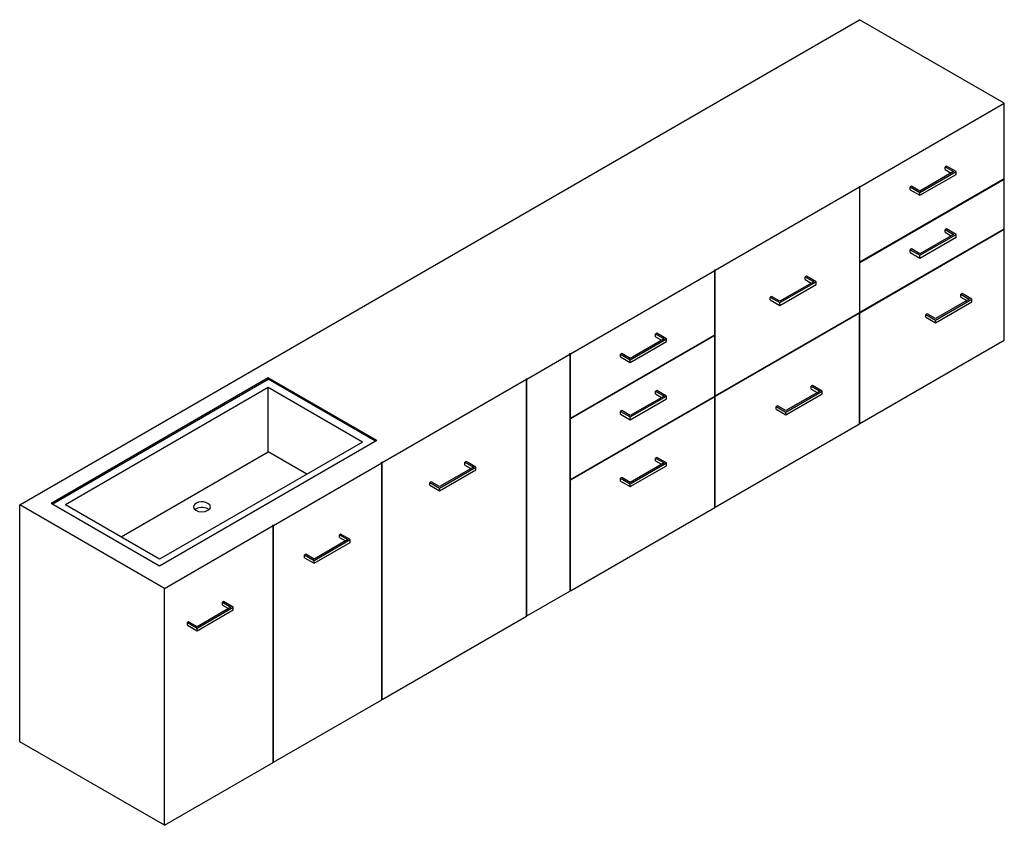
# Model space of a CAD drawing. Units: centimetres. Extents: x 184 to 3717, y -1063 to 1827.
import ezdxf

# ---------------------------------------------------------------- set-up
doc = ezdxf.new("R2010")
doc.units = ezdxf.units.CM
doc.header["$MEASUREMENT"] = 0
doc.layers.add('A-FURN', color=8, linetype='Continuous', lineweight=25)

msp = doc.modelspace()

# ---------------------------------------------------------------- linework, layer by layer
at = {"layer": 'A-FURN'}
for p, q in [((184, 87.1), (3197.8, 1827.1)), ((3717.4, 1527.1), (3197.8, 1827.1)), ((3199.5, 1228.1), (3717.4, 1527.1)), ((3717.4, 1257.1), (3717.4, 1527.1)), ((3414.3, 1207.1), (3544.2, 1282.1)), ((3535.5, 1282.1), (3414.3, 1212.1)), ((3414.3, 1197.1), (3544.2, 1272.1)), ((3509.6, 1302.1), (3505.2, 1299.6)), ((3505.2, 1289.6), (3505.2, 1299.6)), ((3505.2, 1299.6), (3535.5, 1282.1)), ((3505.2, 1289.6), (3526.9, 1277.1)), ((3544.2, 1282.1), (3509.6, 1302.1)), ((3544.2, 1272.1), (3544.2, 1282.1)), ((3199.5, 958.1), (3717.4, 1257.1)), ((3199.5, 956.1), (3717.4, 1255.1)), ((3717.4, 1255.1), (3715.7, 1256.1)), ((3717.4, 1077.1), (3717.4, 1255.1)), ((2679.9, 928.1), (3197.8, 1227.1)), ((3196.1, 1228.1), (3197.8, 1229.1)), ((3197.8, 1227.1), (3196.1, 1228.1)), ((3199.5, 1228.1), (3197.8, 1229.1)), ((3197.8, 1227.1), (3197.8, 1229.1)), ((3197.8, 1227.1), (3197.8, 777.1)), ((3199.5, 958.1), (3199.5, 1228.1)), ((3384, 1229.6), (3379.7, 1227.1)), ((3379.7, 1217.1), (3379.7, 1227.1)), ((3379.7, 1227.1), (3414.3, 1207.1)), ((3379.7, 1217.1), (3414.3, 1197.1)), ((3414.3, 1212.1), (3384, 1229.6)), ((3414.3, 1197.1), (3414.3, 1207.1)), ((3199.5, 778.1), (3717.4, 1077.1)), ((3199.5, 776.1), (3717.4, 1075.1)), ((3509.6, 1077.1), (3505.2, 1074.6)), ((3505.2, 1064.6), (3505.2, 1074.6)), ((3505.2, 1074.6), (3535.5, 1057.1)), ((3505.2, 1064.6), (3526.9, 1052.1)), ((3544.2, 1057.1), (3509.6, 1077.1)), ((3717.4, 1075.1), (3715.7, 1076.1)), ((3717.4, 677.1), (3717.4, 1075.1)), ((3414.3, 982.1), (3544.2, 1057.1)), ((3535.5, 1057.1), (3414.3, 987.1)), ((3414.3, 972.1), (3544.2, 1047.1)), ((3544.2, 1047.1), (3544.2, 1057.1)), ((3384, 1004.6), (3379.7, 1002.1)), ((3379.7, 992.1), (3379.7, 1002.1)), ((3379.7, 1002.1), (3414.3, 982.1)), ((3379.7, 992.1), (3414.3, 972.1)), ((3414.3, 987.1), (3384, 1004.6)), ((3197.8, 959.1), (3199.5, 958.1)), ((3197.8, 957.1), (3199.5, 958.1)), ((3197.8, 957.1), (3199.5, 956.1)), ((3199.5, 778.1), (3199.5, 956.1)), ((3414.3, 972.1), (3414.3, 982.1)), ((2160.3, 628.1), (2678.2, 927.1)), ((2676.5, 928.1), (2678.2, 929.1)), ((2678.2, 927.1), (2676.5, 928.1)), ((2679.9, 928.1), (2678.2, 929.1)), ((2678.2, 927.1), (2678.2, 929.1)), ((2678.2, 697.1), (2678.2, 927.1)), ((2679.9, 478.1), (2679.9, 928.1)), ((2912, 812.1), (3041.9, 887.1)), ((3033.3, 887.1), (2912, 817.1)), ((3007.3, 907.1), (3002.9, 904.6)), ((3002.9, 894.6), (3002.9, 904.6)), ((3002.9, 904.6), (3033.3, 887.1)), ((3002.9, 894.6), (3024.6, 882.1)), ((3041.9, 887.1), (3007.3, 907.1)), ((3041.9, 877.1), (3041.9, 887.1)), ((2912, 802.1), (3041.9, 877.1)), ((2881.7, 834.6), (2877.4, 832.1)), ((2877.4, 822.1), (2877.4, 832.1)), ((2877.4, 832.1), (2912, 812.1)), ((2877.4, 822.1), (2912, 802.1)), ((2912, 817.1), (2881.7, 834.6)), ((3470.6, 749.6), (3600.5, 824.6)), ((3591.8, 824.6), (3470.6, 754.6)), ((3470.6, 739.6), (3600.5, 814.6)), ((3565.9, 844.6), (3561.5, 842.1)), ((3561.5, 832.1), (3561.5, 842.1)), ((3561.5, 842.1), (3591.8, 824.6)), ((3561.5, 832.1), (3583.2, 819.6)), ((3600.5, 824.6), (3565.9, 844.6)), ((3600.5, 814.6), (3600.5, 824.6)), ((2912, 802.1), (2912, 812.1)), ((3197.8, 779.1), (3199.5, 778.1)), ((3197.8, 777.1), (3199.5, 778.1)), ((2679.9, 478.1), (3197.8, 777.1)), ((2679.9, 476.1), (3197.8, 775.1)), ((3196.1, 776.1), (3197.8, 775.1)), ((3197.8, 775.1), (3197.8, 777.1)), ((3197.8, 777.1), (3199.5, 776.1)), ((3197.8, 377.1), (3197.8, 775.1)), ((3199.5, 378.1), (3199.5, 776.1)), ((3440.3, 772.1), (3436, 769.6)), ((3436, 759.6), (3436, 769.6)), ((3436, 769.6), (3470.6, 749.6)), ((3436, 759.6), (3470.6, 739.6)), ((3470.6, 754.6), (3440.3, 772.1)), ((3470.6, 739.6), (3470.6, 749.6)), ((2160.3, 398.1), (2678.2, 697.1)), ((2160.3, 396.1), (2678.2, 695.1)), ((2375.1, 607.1), (2505, 682.1)), ((2496.3, 682.1), (2375.1, 612.1)), ((2375.1, 597.1), (2505, 672.1)), ((2470.3, 702.1), (2466, 699.6)), ((2466, 689.6), (2466, 699.6)), ((2466, 699.6), (2496.3, 682.1)), ((2466, 689.6), (2487.7, 677.1)), ((2505, 682.1), (2470.3, 702.1)), ((2505, 672.1), (2505, 682.1)), ((2678.2, 695.1), (2676.5, 696.1)), ((2678.2, 695.1), (2678.2, 697.1)), ((2678.2, 477.1), (2678.2, 695.1)), ((3199.5, 378.1), (3717.4, 677.1)), ((2004.4, 538.1), (2158.6, 627.1)), ((2156.8, 628.1), (2158.6, 629.1)), ((2158.6, 627.1), (2156.8, 628.1)), ((2160.3, 628.1), (2158.6, 629.1)), ((2158.6, 627.1), (2158.6, 629.1)), ((2158.6, 627.1), (2158.6, -222.9)), ((2160.3, 398.1), (2160.3, 628.1)), ((2344.8, 629.6), (2340.4, 627.1)), ((2340.4, 617.1), (2340.4, 627.1)), ((2340.4, 627.1), (2375.1, 607.1)), ((2340.4, 617.1), (2375.1, 597.1)), ((2375.1, 612.1), (2344.8, 629.6)), ((2375.1, 597.1), (2375.1, 607.1)), ((1076, 542.1), (296.6, 92.1)), ((300.9, 89.6), (1076, 537.1)), ((1465.7, 317.1), (1076, 542.1)), ((1076, 537.1), (1076, 542.1)), ((1461.4, 314.6), (1076, 537.1)), ((1484.8, 238.1), (2002.7, 537.1)), ((2001, 538.1), (2002.7, 539.1)), ((2002.7, 537.1), (2001, 538.1)), ((2004.4, 538.1), (2002.7, 539.1)), ((2002.7, 537.1), (2002.7, 539.1)), ((2002.7, -312.9), (2002.7, 537.1)), ((2004.4, -311.9), (2004.4, 538.1)), ((1076, 507.1), (348.6, 87.1)), ((1413.8, 312.1), (1076, 507.1)), ((1076, 277.1), (1076, 507.1)), ((2470.3, 497.1), (2466, 494.6)), ((2505, 477.1), (2470.3, 497.1)), ((3028.9, 514.6), (3024.6, 512.1)), ((3024.6, 502.1), (3024.6, 512.1)), ((3024.6, 512.1), (3054.9, 494.6)), ((3024.6, 502.1), (3046.2, 489.6)), ((3063.6, 494.6), (3028.9, 514.6)), ((2160.3, 178.1), (2678.2, 477.1)), ((2160.3, 176.1), (2678.2, 475.1)), ((2375.1, 402.1), (2505, 477.1)), ((2496.3, 477.1), (2375.1, 407.1)), ((2375.1, 392.1), (2505, 467.1)), ((2466, 484.6), (2466, 494.6)), ((2466, 494.6), (2496.3, 477.1)), ((2466, 484.6), (2487.7, 472.1)), ((2505, 467.1), (2505, 477.1)), ((2676.5, 476.1), (2678.2, 475.1)), ((2678.2, 479.1), (2679.9, 478.1)), ((2678.2, 477.1), (2679.9, 478.1)), ((2678.2, 475.1), (2678.2, 477.1)), ((2678.2, 477.1), (2679.9, 476.1)), ((2678.2, 77.1), (2678.2, 475.1)), ((2679.9, 78.1), (2679.9, 476.1)), ((2933.7, 419.6), (3063.6, 494.6)), ((3054.9, 494.6), (2933.7, 424.6)), ((2933.7, 409.6), (3063.6, 484.6)), ((3063.6, 484.6), (3063.6, 494.6)), ((2344.8, 424.6), (2340.4, 422.1)), ((2375.1, 407.1), (2344.8, 424.6)), ((2903.4, 442.1), (2899, 439.6)), ((2899, 429.6), (2899, 439.6)), ((2899, 439.6), (2933.7, 419.6)), ((2899, 429.6), (2933.7, 409.6)), ((2933.7, 424.6), (2903.4, 442.1)), ((2158.6, 399.1), (2160.3, 398.1)), ((2158.6, 397.1), (2160.3, 398.1)), ((2158.6, 397.1), (2160.3, 396.1)), ((2160.3, 178.1), (2160.3, 396.1)), ((2340.4, 412.1), (2340.4, 422.1)), ((2340.4, 422.1), (2375.1, 402.1)), ((2340.4, 412.1), (2375.1, 392.1)), ((2375.1, 392.1), (2375.1, 402.1)), ((2933.7, 409.6), (2933.7, 419.6)), ((2679.9, 78.1), (3197.8, 377.1)), ((3199.5, 378.1), (3197.8, 379.1)), ((1465.7, 317.1), (686.3, -132.9)), ((1413.8, 312.1), (686.3, -107.9)), ((547.8, -27.9), (1076, 277.1)), ((1214.6, 197.1), (1076, 277.1)), ((2470.3, 257.1), (2466, 254.6)), ((2466, 244.6), (2466, 254.6)), ((2466, 254.6), (2496.3, 237.1)), ((2505, 237.1), (2470.3, 257.1)), ((1095.1, 13.1), (1483.1, 237.1)), ((1481.3, 238.1), (1483.1, 239.1)), ((1483.1, 237.1), (1481.3, 238.1)), ((1484.8, 238.1), (1483.1, 239.1)), ((1483.1, 237.1), (1483.1, 239.1)), ((1483.1, -612.9), (1483.1, 237.1)), ((1484.8, -611.9), (1484.8, 238.1)), ((1690.9, 147.1), (1820.8, 222.1)), ((1812.2, 222.1), (1690.9, 152.1)), ((1690.9, 137.1), (1820.8, 212.1)), ((1786.2, 242.1), (1781.8, 239.6)), ((1781.8, 229.6), (1781.8, 239.6)), ((1781.8, 239.6), (1812.2, 222.1)), ((1781.8, 229.6), (1803.5, 217.1)), ((1820.8, 222.1), (1786.2, 242.1)), ((1820.8, 212.1), (1820.8, 222.1)), ((2375.1, 162.1), (2505, 237.1)), ((2496.3, 237.1), (2375.1, 167.1)), ((2375.1, 152.1), (2505, 227.1)), ((2466, 244.6), (2487.7, 232.1)), ((2505, 227.1), (2505, 237.1)), ((2158.6, 179.1), (2160.3, 178.1)), ((2158.6, 177.1), (2160.3, 178.1)), ((2158.6, 177.1), (2160.3, 176.1)), ((2344.8, 184.6), (2340.4, 182.1)), ((2340.4, 172.1), (2340.4, 182.1)), ((2340.4, 182.1), (2375.1, 162.1)), ((2375.1, 167.1), (2344.8, 184.6)), ((1660.6, 169.6), (1656.3, 167.1)), ((1656.3, 157.1), (1656.3, 167.1)), ((1656.3, 167.1), (1690.9, 147.1)), ((1656.3, 157.1), (1690.9, 137.1)), ((1690.9, 152.1), (1660.6, 169.6)), ((1690.9, 137.1), (1690.9, 147.1)), ((2160.3, -221.9), (2160.3, 176.1)), ((2340.4, 172.1), (2375.1, 152.1)), ((2375.1, 152.1), (2375.1, 162.1)), ((703.6, -212.9), (184, 87.1)), ((184, -762.9), (184, 87.1)), ((686.3, -132.9), (296.6, 92.1)), ((686.3, -107.9), (348.6, 87.1)), ((2160.3, -221.9), (2678.2, 77.1)), ((2679.9, 78.1), (2678.2, 79.1)), ((703.6, -212.9), (1093.4, 12.1)), ((1091.6, 13.1), (1093.4, 14.1)), ((1093.4, 12.1), (1091.6, 13.1)), ((1095.1, 13.1), (1093.4, 14.1)), ((1093.4, 12.1), (1093.4, 14.1)), ((1093.4, -837.9), (1093.4, 12.1)), ((1095.1, -836.9), (1095.1, 13.1)), ((1335.8, -17.9), (1331.5, -20.4)), ((1331.5, -30.4), (1331.5, -20.4)), ((1331.5, -20.4), (1361.8, -37.9)), ((1331.5, -30.4), (1353.2, -42.9)), ((1370.5, -37.9), (1335.8, -17.9)), ((1240.6, -112.9), (1370.5, -37.9)), ((1361.8, -37.9), (1240.6, -107.9)), ((1240.6, -122.9), (1370.5, -47.9)), ((1370.5, -47.9), (1370.5, -37.9)), ((1210.3, -90.4), (1205.9, -92.9)), ((1205.9, -102.9), (1205.9, -92.9)), ((1205.9, -92.9), (1240.6, -112.9)), ((1205.9, -102.9), (1240.6, -122.9)), ((1240.6, -107.9), (1210.3, -90.4)), ((1240.6, -122.9), (1240.6, -112.9)), ((703.6, -1062.9), (703.6, -212.9)), ((2004.4, -311.9), (2158.6, -222.9)), ((2160.3, -221.9), (2158.6, -220.9)), ((820.6, -355.4), (950.5, -280.4)), ((941.8, -280.4), (820.6, -350.4)), ((915.8, -260.4), (911.5, -262.9)), ((911.5, -272.9), (911.5, -262.9)), ((911.5, -262.9), (941.8, -280.4)), ((911.5, -272.9), (933.1, -285.4)), ((950.5, -280.4), (915.8, -260.4)), ((950.5, -290.4), (950.5, -280.4)), ((820.6, -365.4), (950.5, -290.4)), ((1484.8, -611.9), (2002.7, -312.9)), ((2004.4, -311.9), (2002.7, -310.9)), ((790.2, -332.9), (785.9, -335.4)), ((785.9, -345.4), (785.9, -335.4)), ((785.9, -335.4), (820.6, -355.4)), ((785.9, -345.4), (820.6, -365.4)), ((820.6, -350.4), (790.2, -332.9)), ((820.6, -365.4), (820.6, -355.4)), ((1095.1, -836.9), (1483.1, -612.9)), ((1484.8, -611.9), (1483.1, -610.9)), ((703.6, -1062.9), (184, -762.9)), ((703.6, -1062.9), (1093.4, -837.9)), ((1095.1, -836.9), (1093.4, -835.9))]:
    msp.add_line(p, q, dxfattribs=at)
for centre, start_param, end_param in [((837.9, 79.6), 0.785398, 3.141593), ((837.9, 79.6), 3.141593, 6.283185), ((837.9, 59.6), 0.785398, 2.540328), ((837.9, 79.6), 0, 0.785398), ((837.9, 59.6), 0.601264, 0.785398)]:
    msp.add_ellipse(centre, major_axis=(30.6, 0), ratio=0.57735, start_param=start_param, end_param=end_param, dxfattribs=at)

doc.saveas('drawing.dxf')
